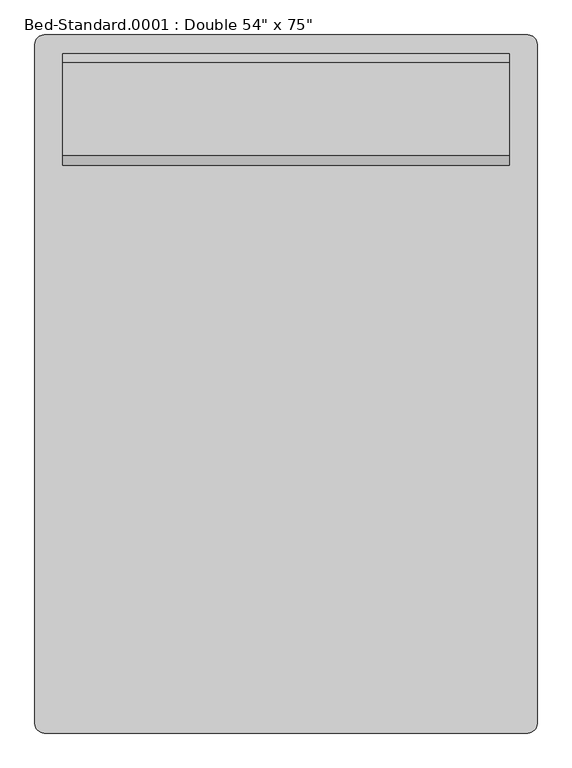
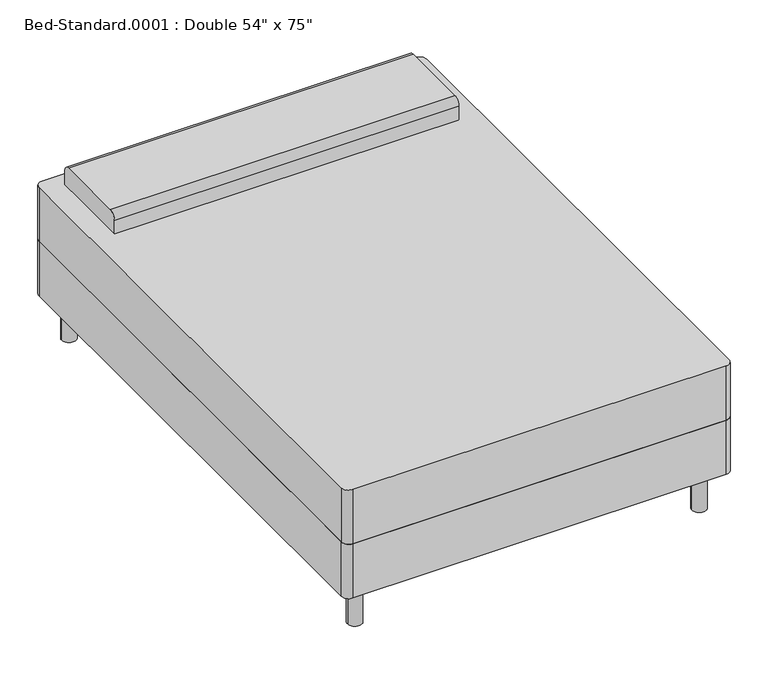
"""IFC4 building model written with IfcOpenShell, lengths in millimetres: furniture geometry."""

from ifc_helpers import new_model, si_unit, point, frame, frame_2d, origin, origin_with_axes, place, context, project, spatial, polyline, circle_curve, trimmed, segment, composite_curve, outline, extrude, source, transform, mapped, element, save


def furniture_0253826f(model_context):
    return source(origin(), model_context, "Body", "SweptSolid", [
        extrude(outline(composite_curve([segment(polyline([(-414.3114754, -972.695082), (-414.3114754, 881.504918)]), True, "CONTINUOUS"), segment(trimmed(circle_curve(frame_2d((-388.9114754, 881.504918)), 25.4), [point((-414.3114754, 881.504918))], [point((-388.9114754, 906.904918))], False, "CARTESIAN"), True, "CONTINUOUS"), segment(polyline([(-388.9114754, 906.904918), (931.8885246, 906.904918)]), True, "CONTINUOUS"), segment(trimmed(circle_curve(frame_2d((931.8885246, 881.504918)), 25.4), [point((931.8885246, 906.904918))], [point((957.2885246, 881.504918))], False, "CARTESIAN"), True, "CONTINUOUS"), segment(polyline([(957.2885246, 881.504918), (957.2885246, -972.695082)]), True, "CONTINUOUS"), segment(trimmed(circle_curve(frame_2d((931.8885246, -972.695082)), 25.4), [point((957.2885246, -972.695082))], [point((931.8885246, -998.095082))], False, "CARTESIAN"), True, "CONTINUOUS"), segment(polyline([(931.8885246, -998.095082), (-388.9114754, -998.095082)]), True, "CONTINUOUS"), segment(trimmed(circle_curve(frame_2d((-388.9114754, -972.695082)), 25.4), [point((-388.9114754, -998.095082))], [point((-414.3114754, -972.695082))], False, "CARTESIAN"), True, "CONTINUOUS")], self_intersect=False)), frame((0.0, 0.0, 152.4), z_axis=(0.0, 0.0, 1.0), x_axis=(1.0, 0.0, 0.0)), (0.0, 0.0, 1.0), 203.2),
        extrude(outline(composite_curve([segment(polyline([(551.304918, 558.8), (551.304918, 609.6)]), True, "CONTINUOUS"), segment(trimmed(circle_curve(frame_2d((576.704918, 609.6)), 25.4), [point((551.304918, 609.6))], [point((576.704918, 635.0))], False, "CARTESIAN"), True, "CONTINUOUS"), segment(polyline([(576.704918, 635.0), (830.704918, 635.0)]), True, "CONTINUOUS"), segment(trimmed(circle_curve(frame_2d((830.704918, 609.6)), 25.4), [point((830.704918, 635.0))], [point((856.104918, 609.6))], False, "CARTESIAN"), True, "CONTINUOUS"), segment(polyline([(856.104918, 609.6), (856.104918, 558.8), (551.304918, 558.8)]), True, "CONTINUOUS")], self_intersect=False)), frame((-338.1114754, 0.0, 0.0), z_axis=(1.0, 0.0, 0.0), x_axis=(0.0, 1.0, 0.0)), (0.0, 0.0, 1.0), 1219.2),
        extrude(outline(composite_curve([segment(trimmed(circle_curve(frame_2d((-338.1114754, 830.704918)), 25.4), [point((-363.5114754, 830.704918))], [point((-312.7114754, 830.704918))], False, "CARTESIAN"), True, "CONTINUOUS"), segment(trimmed(circle_curve(frame_2d((-338.1114754, 830.704918)), 25.4), [point((-312.7114754, 830.704918))], [point((-363.5114754, 830.704918))], False, "CARTESIAN"), True, "CONTINUOUS")], self_intersect=False)), origin_with_axes(), (0.0, 0.0, 1.0), 152.4),
        extrude(outline(composite_curve([segment(trimmed(circle_curve(frame_2d((881.0885246, 830.704918)), 25.4), [point((855.6885246, 830.704918))], [point((906.4885246, 830.704918))], False, "CARTESIAN"), True, "CONTINUOUS"), segment(trimmed(circle_curve(frame_2d((881.0885246, 830.704918)), 25.4), [point((906.4885246, 830.704918))], [point((855.6885246, 830.704918))], False, "CARTESIAN"), True, "CONTINUOUS")], self_intersect=False)), origin_with_axes(), (0.0, 0.0, 1.0), 152.4),
        extrude(outline(composite_curve([segment(trimmed(circle_curve(frame_2d((881.0885246, -921.895082)), 25.4), [point((855.6885246, -921.895082))], [point((906.4885246, -921.895082))], False, "CARTESIAN"), True, "CONTINUOUS"), segment(trimmed(circle_curve(frame_2d((881.0885246, -921.895082)), 25.4), [point((906.4885246, -921.895082))], [point((855.6885246, -921.895082))], False, "CARTESIAN"), True, "CONTINUOUS")], self_intersect=False)), origin_with_axes(), (0.0, 0.0, 1.0), 152.4),
        extrude(outline(composite_curve([segment(trimmed(circle_curve(frame_2d((-338.1114754, -921.895082)), 25.4), [point((-363.5114754, -921.895082))], [point((-312.7114754, -921.895082))], False, "CARTESIAN"), True, "CONTINUOUS"), segment(trimmed(circle_curve(frame_2d((-338.1114754, -921.895082)), 25.4), [point((-312.7114754, -921.895082))], [point((-363.5114754, -921.895082))], False, "CARTESIAN"), True, "CONTINUOUS")], self_intersect=False)), origin_with_axes(), (0.0, 0.0, 1.0), 152.4),
        extrude(outline(composite_curve([segment(polyline([(-388.9114754, 906.904918), (931.8885246, 906.904918)]), True, "CONTINUOUS"), segment(trimmed(circle_curve(frame_2d((931.8885246, 881.504918)), 25.4), [point((931.8885246, 906.904918))], [point((957.2885246, 881.504918))], False, "CARTESIAN"), True, "CONTINUOUS"), segment(polyline([(957.2885246, 881.504918), (957.2885246, -972.695082)]), True, "CONTINUOUS"), segment(trimmed(circle_curve(frame_2d((931.8885246, -972.695082)), 25.4), [point((957.2885246, -972.695082))], [point((931.8885246, -998.095082))], False, "CARTESIAN"), True, "CONTINUOUS"), segment(polyline([(931.8885246, -998.095082), (-388.9114754, -998.095082)]), True, "CONTINUOUS"), segment(trimmed(circle_curve(frame_2d((-388.9114754, -972.695082)), 25.4), [point((-388.9114754, -998.095082))], [point((-414.3114754, -972.695082))], False, "CARTESIAN"), True, "CONTINUOUS"), segment(polyline([(-414.3114754, -972.695082), (-414.3114754, 881.504918)]), True, "CONTINUOUS"), segment(trimmed(circle_curve(frame_2d((-388.9114754, 881.504918)), 25.4), [point((-414.3114754, 881.504918))], [point((-388.9114754, 906.904918))], False, "CARTESIAN"), True, "CONTINUOUS")], self_intersect=False)), frame((0.0, 0.0, 355.6), z_axis=(0.0, 0.0, 1.0), x_axis=(1.0, 0.0, 0.0)), (0.0, 0.0, 1.0), 203.2),
    ])


if __name__ == "__main__":
    model = new_model("IFC4")
    model_context = context("Model", 3, world=origin())
    ifc_project = project(units=[si_unit("LENGTHUNIT", "METRE", prefix="MILLI")], contexts=[model_context])
    site = spatial("IfcSite", under=ifc_project)
    building = spatial("IfcBuilding", under=site)
    placement = place(None, origin())
    furniture_shape = furniture_0253826f(model_context)
    element("IfcFurniture", 1, ObjectType="Bed-Standard.0001 : Double 54\" x 75\"", at=placement, inside=building, context=model_context, shape_type="MappedRepresentation", body=[
        mapped(furniture_shape, transform((0.0, 0.0, 0.0), x_axis=(1.0, 0.0, 0.0), y_axis=(0.0, 1.0, 0.0), z_axis=(0.0, 0.0, 1.0))),
    ])
    save(model, "model.ifc")

# Revit data of these elements
# Type "Bed-Standard.0001 : Double 54\" x 75\""
#   Assembly Code = "E2020200"
#   Length = 6' - 3"
#   Width = 4' - 6"
#   Leg Material = Steel, Chrome Plated
#   Mattress Material = Plywood, Sheathing
#   Default Elevation = 0
# Element 1 (IfcFurniture, "Bed-Standard.0001 : Double 54\" x 75\"")
#   Materials on its faces: "Linen, White", "Steel, Chrome Plated"
# Materials
#   "Steel, Chrome Plated": class "Metal", colour RGB 17 17 17, transparency 0, Description = "Chromiuim plated steel", Cost = 0
#   "Plywood, Sheathing": class "Wood", colour RGB 212 179 113, transparency 0, Description = "Plywood, sheathing grade", Cost = 0
#   "Linen, White": class "Textile", colour RGB 247 247 239, transparency 0, Description = "Linen, white", Cost = 0
